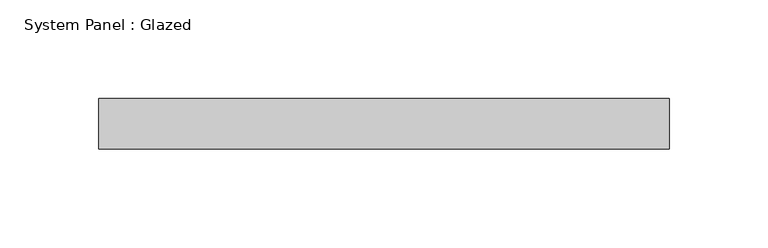
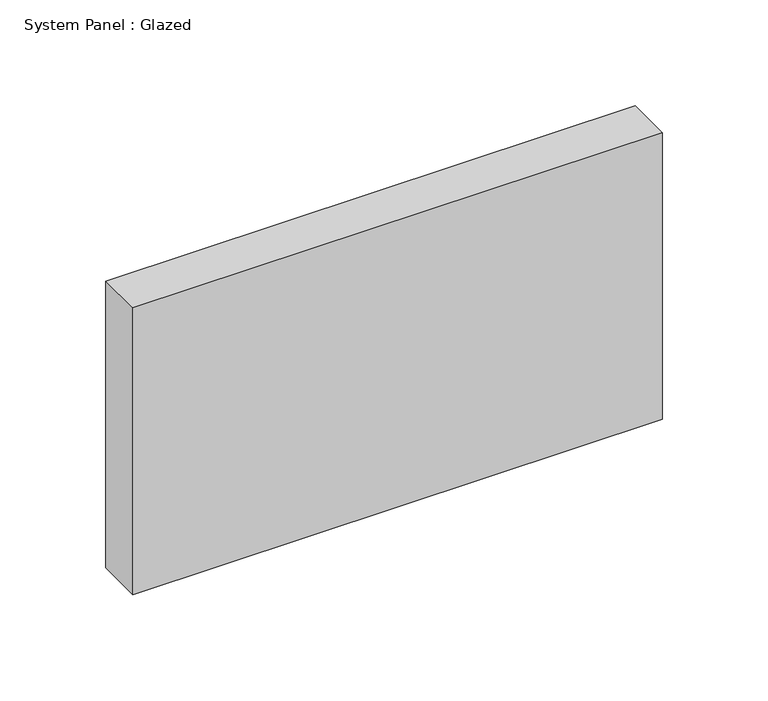
"""IFC4 building model written with IfcOpenShell, lengths in millimetres: plate geometry, System Panel : Glazed."""

from ifc_helpers import new_model, si_unit, origin, origin_with_axes, place, context, project, spatial, polyline, outline, extrude, source, transform, mapped, element, save


def system_panel_glazed_e426d894(model_context):
    return source(origin(), model_context, "Body", "SweptSolid", [
        extrude(outline(polyline([(144.1160334, 19.05), (-144.1160334, 19.05), (-144.1160334, 44.45), (144.1160334, 44.45), (144.1160334, 19.05)])), origin_with_axes(), (0.0, 0.0, 1.0), 165.1),
    ])


if __name__ == "__main__":
    model = new_model("IFC4")
    model_context = context("Model", 3, world=origin())
    ifc_project = project(units=[si_unit("LENGTHUNIT", "METRE", prefix="MILLI")], contexts=[model_context])
    site = spatial("IfcSite", under=ifc_project)
    building = spatial("IfcBuilding", under=site)
    placement = place(None, origin())
    system_panel_glazed_shape = system_panel_glazed_e426d894(model_context)
    element("IfcPlate", 1, ObjectType="System Panel : Glazed", at=placement, inside=building, context=model_context, shape_type="MappedRepresentation", body=[
        mapped(system_panel_glazed_shape, transform((0.0, 0.0, 0.0), x_axis=(1.0, 0.0, 0.0), y_axis=(0.0, 1.0, 0.0), z_axis=(0.0, 0.0, 1.0))),
    ])
    save(model, "model.ifc")

# Revit data of these elements
# Type "System Panel : Glazed"
#   Construction Type Id = "GSP4R"
#   Analytic Construction = "1/8 in Pilkington single glazing"
#   Visual Light Transmittance = 0.9
#   Solar Heat Gain Coefficient = 0.86
#   Heat Transfer Coefficient (U) = 1.18115 BTU/(h·ft²·°F)
#   Define Thermal Properties by = 1
# Element 1 (IfcPlate, "System Panel : Glazed")
#   Materials on its faces: "Glass"
# Materials
#   "Glass": class "Glass", colour RGB 0 128 192, transparency 0.75, Description = "Soda Lime Glass", Cost = 0
